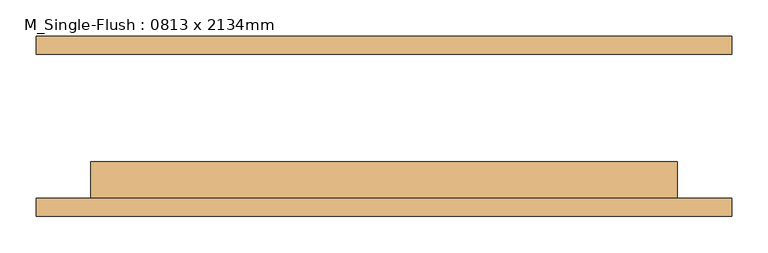
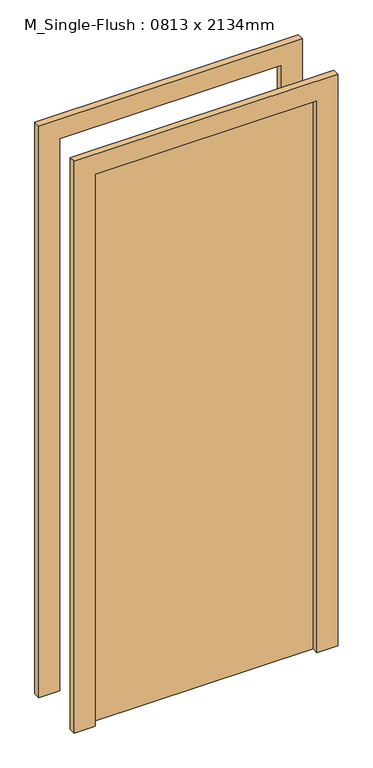
"""IFC4 building model written with IfcOpenShell, lengths in millimetres: door geometry, M_Single-Flush : 0813 x 2134mm."""

from ifc_helpers import new_model, si_unit, frame, origin, origin_with_axes, place, context, project, spatial, polyline, outline, extrude, source, transform, mapped, element, save


def m_single_flush_0813_x_2134mm_c8a1819b(model_context):
    return source(origin(), model_context, "Body", "SweptSolid", [
        extrude(outline(polyline([(2210.0, -482.5), (0.0, -482.5), (0.0, -406.5), (2134.0, -406.5), (2134.0, 406.5), (0.0, 406.5), (0.0, 482.5), (2210.0, 482.5), (2210.0, -482.5)])), frame((0.0, -125.0, 0.0), z_axis=(0.0, 1.0, 0.0), x_axis=(0.0, 0.0, 1.0)), (0.0, 0.0, 1.0), 25.0),
        extrude(outline(polyline([(2210.0, 482.5), (2210.0, -482.5), (0.0, -482.5), (0.0, -406.5), (2134.0, -406.5), (2134.0, 406.5), (0.0, 406.5), (0.0, 482.5), (2210.0, 482.5)])), frame((0.0, 100.0, 0.0), z_axis=(0.0, 1.0, 0.0), x_axis=(0.0, 0.0, 1.0)), (0.0, 0.0, 1.0), 25.0),
        extrude(outline(polyline([(406.5, -49.0), (406.5, -100.0), (-406.5, -100.0), (-406.5, -49.0), (406.5, -49.0)])), origin_with_axes(), (0.0, 0.0, 1.0), 2134.0),
    ])


if __name__ == "__main__":
    model = new_model("IFC4")
    model_context = context("Model", 3, world=origin())
    ifc_project = project(units=[si_unit("LENGTHUNIT", "METRE", prefix="MILLI")], contexts=[model_context])
    site = spatial("IfcSite", under=ifc_project)
    building = spatial("IfcBuilding", under=site)
    placement = place(None, origin())
    m_single_flush_0813_x_2134mm_shape = m_single_flush_0813_x_2134mm_c8a1819b(model_context)
    element("IfcDoor", 1, ObjectType="M_Single-Flush : 0813 x 2134mm", at=placement, inside=building, context=model_context, shape_type="MappedRepresentation", body=[
        mapped(m_single_flush_0813_x_2134mm_shape, transform((0.0, 0.0, 0.0), x_axis=(1.0, 0.0, 0.0), y_axis=(0.0, 1.0, 0.0), z_axis=(0.0, 0.0, 1.0))),
    ])
    save(model, "model.ifc")

# Revit data of these elements
# Type "M_Single-Flush : 0813 x 2134mm"
#   Type Mark = "17"
#   Thickness = 51 mm
#   Height = 2134 mm
#   Trim Projection Ext = 25 mm
#   Trim Projection Int = 25 mm
#   Trim Width = 76 mm
#   Width = 813 mm
#   Door Material = Door - Panel
#   Frame Material = Door - Frame
#   Function = (empty or 0)
#   Wall Closure = (empty or 0)
# Element 1 (IfcDoor, "M_Single-Flush : 0813 x 2134mm")
#   Materials on its faces: "Door - Frame", "Door - Panel"
# Materials
#   "Door - Panel": class "Wood", colour RGB 114 82 51, transparency 0
#   "Door - Frame": colour RGB 153 76 43, transparency 0
